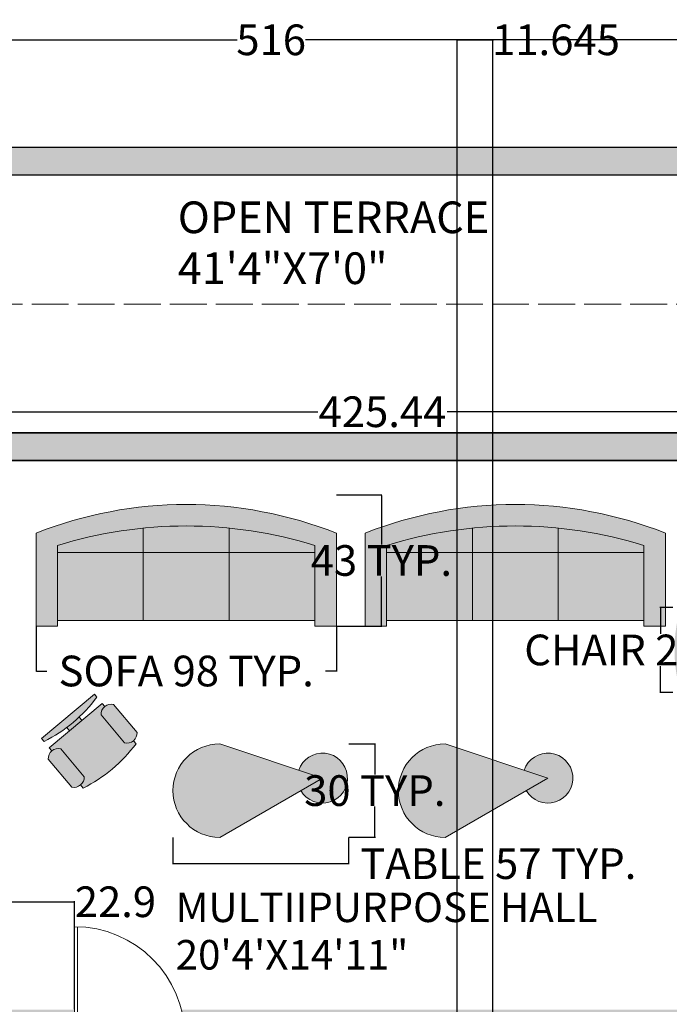
# Model space of a CAD drawing. Units: inches. Extents: x 409 to 1056, y 160 to 945.
# Tile 5 of 6: x 632 to 843, y 624 to 945. Entities that reach past the tile are written whole.
import ezdxf

# ---------------------------------------------------------------- set-up
doc = ezdxf.new("R2010")
doc.units = ezdxf.units.IN
doc.header["$MEASUREMENT"] = 0
doc.linetypes.add('ACAD_ISO02W100', pattern=[15, 12, -3])
for name, color, linetype, lineweight in [('A-ANNO-DIMS', 2, 'Continuous', 18), ('A-AREA-IDEN', 7, 'Continuous', 18), ('A-DOOR', 3, 'Continuous', 18), ('A-FURN', 8, 'Continuous', 18), ('A-ROOF-BYND', 8, 'ACAD_ISO02W100', 13), ('A-WALL', 7, 'Continuous', 35), ('A-WALL-PRPT', 7, 'Continuous', 30)]:
    doc.layers.add(name, color=color, linetype=linetype, lineweight=lineweight)
doc.layers.add('A-FURN-PATT', color=51, linetype='Continuous', lineweight=13, true_color=0xf8f6b0)
doc.layers.add('A-WALL-PATT', color=251, linetype='Continuous', lineweight=13, true_color=0x636466)
doc.styles.get("Standard").update_dxf_attribs({"font": 'arial.ttf'})
doc.dimstyles.get("Standard").update_dxf_attribs({"dimtxt": 10, "dimasz": 0.18, "dimexe": 0.18, "dimexo": 0.0625, "dimgap": 0.09, "dimtad": 0, "dimtih": 1, "dimtoh": 1, "dimdec": 0, "dimzin": 0, "dimdsep": 46, "dimlunit": 3, "dimtxsty": 'Standard', "dimcen": 0.09, "dimadec": 0, "dimazin": 0, "dimtfac": 1, "dimtdec": 0, "dimtofl": 0, "dimtmove": 0, "dimatfit": 3, "dimfxl": 1, "dimtolj": 1, "dimtzin": 0, "dimarcsym": 0})

# ---------------------------------------------------------------- blocks, each defined once
blk = doc.blocks.new('Sofa - Roundback 7 ft.')
for p, q in [((-12.00002, -32.4421), (-12.00003, -6.5971)), ((11.99997, -32.4421), (11.99998, -6.5971)), ((-36.000027, -34), (-36.000027, -11.4696)), ((-35.999844, -13.3819), (35.9998, -13.3819)), ((35.99998, -34), (35.99998, -11.4696)), ((-36.000027, -32.4421), (35.99998, -32.4421))]:
    blk.add_line(p, q)
for points in [[(-36.000027, -34), (-42.000027, -34), (-42.000027, -8)], [(41.99998, -8), (41.99998, -34), (35.99998, -34)]]:
    blk.add_lwpolyline(points)
for centre, radius, start, end in [((0, -114.25), 114.25, 68.43141, 111.5686), ((-0.00001, -127.1968), 121.1968, 72.72033, 107.2797)]:
    blk.add_arc(centre, radius, start, end)
blk = doc.blocks.new('Chair - Desk')
for p, q in [((-8.5, 0), (-8.5, -1)), ((-8.5, 0), (8.5, 0)), ((8.5, 0), (8.5, -1)), ((-2, -3), (-2, -1.9355)), ((2, -1.9576), (2, -3)), ((-8.5, -3), (-8.5, -4)), ((-8.5, -3), (8.5, -3)), ((8.5, -3), (8.5, -4)), ((-10.5, -5), (-10.5, -14)), ((-6.5, -14), (-6.5, -5)), ((6.5, -5), (6.5, -14)), ((10.5, -14), (10.5, -5)), ((-8.5, -15), (-8.5, -16)), ((8.5, -15), (8.5, -16))]:
    blk.add_line(p, q)
for centre, radius, start, end in [((0, 34.625), 36.625, 256.5803, 283.4197), ((-8.5, -6.5), 2.5, 36.8699, 143.1301), ((8.5, -6.5), 2.5, 36.8699, 143.1301), ((-8.5, -12.5), 2.5, 216.8699, 323.1301), ((8.5, -12.5), 2.5, 216.8699, 323.1301), ((0, 19.625), 36.625, 256.5803, 283.4197)]:
    blk.add_arc(centre, radius, start, end)
blk = doc.blocks.new('DOOR-SWING-36IN')
for p, q in [((35, 36), (35, 0)), ((36, 36), (36, 0))]:
    blk.add_line(p, q)
blk.add_arc((36, 36), 36, 180, 270)
blk = doc.blocks.new('TABLE-HALL-ACCENT')
for q in [(15.23, 30.46), (15.23, 0)]:
    blk.add_line((48.7, 19.32), q)
for centre, radius, start, end in [((15.23, 15.23), 15.23, 90, 270), ((48.7, 19.32), 8.14, 210, 161.5857)]:
    blk.add_arc(centre, radius, start, end)
blk = doc.blocks.new('*D19')
at = {"layer": 'A-ANNO-DIMS', "color": 0, "lineweight": -2, "transparency": 16777216}
for p, q in [((844.66, 753.84), (840.37, 753.84)), ((840.55, 753.66), (840.55, 745.22)), ((840.55, 726.25), (840.55, 734.7)), ((844.66, 726.07), (840.37, 726.07))]:
    blk.add_line(p, q, dxfattribs=at)
at = {"layer": 'A-ANNO-DIMS', "color": 0, "transparency": 16777216}
for points in [[(840.52, 753.66), (840.58, 753.66), (840.55, 753.84)], [(840.52, 726.25), (840.58, 726.25), (840.55, 726.07)]]:
    blk.add_solid(points, dxfattribs=at)
at = {"layer": 'Defpoints', "color": 0, "transparency": 16777216}
for p in [(844.72, 753.84), (840.55, 726.07), (844.72, 726.07)]:
    blk.add_point(p, dxfattribs=at)
at = {"layer": 'A-ANNO-DIMS', "color": 0, "transparency": 16777216, "insert": (840.55, 739.96), "char_height": 10, "attachment_point": 5}
blk.add_mtext('\\A1;CHAIR 28 TYP.', dxfattribs=at)
blk = doc.blocks.new('*D21')
at = {"layer": 'A-ANNO-DIMS', "color": 0, "lineweight": -2, "transparency": 16777216}
for p, q in [((637.14, 747.71), (637.14, 732.92)), ((734.98, 747.71), (734.98, 732.92)), ((637.32, 733.1), (640.69, 733.1)), ((734.8, 733.1), (731.42, 733.1))]:
    blk.add_line(p, q, dxfattribs=at)
at = {"layer": 'A-ANNO-DIMS', "color": 0, "transparency": 16777216}
for points in [[(637.32, 733.13), (637.32, 733.07), (637.14, 733.1)], [(734.8, 733.13), (734.8, 733.07), (734.98, 733.1)]]:
    blk.add_solid(points, dxfattribs=at)
at = {"layer": 'Defpoints', "color": 0, "transparency": 16777216}
for p in [(637.14, 747.77), (734.98, 747.77), (734.98, 733.1)]:
    blk.add_point(p, dxfattribs=at)
at = {"layer": 'A-ANNO-DIMS', "color": 0, "transparency": 16777216, "insert": (686.06, 733.1), "char_height": 10, "attachment_point": 5}
blk.add_mtext('\\A1;SOFA 98 TYP.', dxfattribs=at)
blk = doc.blocks.new('*D22')
at = {"layer": 'A-ANNO-DIMS', "color": 0, "lineweight": -2, "transparency": 16777216}
for p, q in [((735.04, 790.48), (749.83, 790.48)), ((749.65, 790.3), (749.65, 774.33)), ((749.65, 747.95), (749.65, 763.93)), ((735.04, 747.77), (749.83, 747.77))]:
    blk.add_line(p, q, dxfattribs=at)
at = {"layer": 'A-ANNO-DIMS', "color": 0, "transparency": 16777216}
for points in [[(749.62, 790.3), (749.68, 790.3), (749.65, 790.48)], [(749.62, 747.95), (749.68, 747.95), (749.65, 747.77)]]:
    blk.add_solid(points, dxfattribs=at)
at = {"layer": 'Defpoints', "color": 0, "transparency": 16777216}
for p in [(734.98, 790.48), (749.65, 790.48), (734.98, 747.77)]:
    blk.add_point(p, dxfattribs=at)
at = {"layer": 'A-ANNO-DIMS', "color": 0, "transparency": 16777216, "insert": (749.65, 769.13), "char_height": 10, "attachment_point": 5}
blk.add_mtext('\\A1;43 TYP.', dxfattribs=at)
blk = doc.blocks.new('*D23')
at = {"layer": 'A-ANNO-DIMS', "color": 0, "lineweight": -2, "transparency": 16777216}
for p, q in [((681.75, 678.81), (681.75, 670.12)), ((738.93, 678.81), (738.93, 670.12)), ((681.93, 670.3), (738.75, 670.3)), ((738.93, 670.3), (739.11, 670.3))]:
    blk.add_line(p, q, dxfattribs=at)
at = {"layer": 'A-ANNO-DIMS', "color": 0, "transparency": 16777216}
for points in [[(681.93, 670.33), (681.93, 670.27), (681.75, 670.3)], [(738.75, 670.33), (738.75, 670.27), (738.93, 670.3)]]:
    blk.add_solid(points, dxfattribs=at)
at = {"layer": 'Defpoints', "color": 0, "transparency": 16777216}
for p in [(681.75, 678.88), (738.93, 678.88), (738.93, 670.3)]:
    blk.add_point(p, dxfattribs=at)
at = {"layer": 'A-ANNO-DIMS', "color": 0, "transparency": 16777216, "insert": (787.74, 670.3), "char_height": 10, "attachment_point": 5}
blk.add_mtext('\\A1;TABLE 57 TYP.', dxfattribs=at)
blk = doc.blocks.new('*D24')
at = {"layer": 'A-ANNO-DIMS', "color": 0, "lineweight": -2, "transparency": 16777216}
for p, q in [((739, 709.34), (747.69, 709.34)), ((747.51, 709.16), (747.51, 699.31)), ((747.51, 679.06), (747.51, 688.91)), ((739, 678.88), (747.69, 678.88))]:
    blk.add_line(p, q, dxfattribs=at)
at = {"layer": 'A-ANNO-DIMS', "color": 0, "transparency": 16777216}
for points in [[(747.48, 709.16), (747.54, 709.16), (747.51, 709.34)], [(747.48, 679.06), (747.54, 679.06), (747.51, 678.88)]]:
    blk.add_solid(points, dxfattribs=at)
at = {"layer": 'Defpoints', "color": 0, "transparency": 16777216}
for p in [(738.93, 709.34), (747.51, 709.34), (738.93, 678.88)]:
    blk.add_point(p, dxfattribs=at)
at = {"layer": 'A-ANNO-DIMS', "color": 0, "transparency": 16777216, "insert": (747.51, 694.11), "char_height": 10, "attachment_point": 5}
blk.add_mtext('\\A1;30 TYP.', dxfattribs=at)
blk = doc.blocks.new('*D35')
at = {"layer": 'A-ANNO-DIMS', "color": 0, "lineweight": -2, "transparency": 16777216}
for p, q in [((455.74, 903.81), (455.74, 939.05)), ((455.92, 938.87), (702.61, 938.87)), ((971.56, 938.87), (724.88, 938.87)), ((971.74, 903.81), (971.74, 939.05))]:
    blk.add_line(p, q, dxfattribs=at)
at = {"layer": 'A-ANNO-DIMS', "color": 0, "transparency": 16777216}
for points in [[(455.92, 938.9), (455.92, 938.84), (455.74, 938.87)], [(971.56, 938.9), (971.56, 938.84), (971.74, 938.87)]]:
    blk.add_solid(points, dxfattribs=at)
at = {"layer": 'Defpoints', "color": 0, "transparency": 16777216}
for p in [(971.74, 938.87), (455.74, 903.74), (971.74, 903.74)]:
    blk.add_point(p, dxfattribs=at)
at = {"layer": 'A-ANNO-DIMS', "color": 0, "transparency": 16777216, "insert": (713.74, 938.87), "char_height": 10, "attachment_point": 5}
blk.add_mtext('\\A1;516', dxfattribs=at)
blk = doc.blocks.new('*D53')
at = {"layer": 'A-ANNO-DIMS', "color": 0, "lineweight": -2, "transparency": 16777216}
for p, q in [((774.31, 452.81), (774.31, 939.05)), ((774.49, 938.87), (785.78, 938.87)), ((785.96, 452.81), (785.96, 939.05)), ((785.96, 938.87), (786.14, 938.87))]:
    blk.add_line(p, q, dxfattribs=at)
at = {"layer": 'A-ANNO-DIMS', "color": 0, "transparency": 16777216}
for points in [[(774.49, 938.9), (774.49, 938.84), (774.31, 938.87)], [(785.78, 938.9), (785.78, 938.84), (785.96, 938.87)]]:
    blk.add_solid(points, dxfattribs=at)
at = {"layer": 'Defpoints', "color": 0, "transparency": 16777216}
for p in [(785.96, 938.87), (774.31, 452.74), (785.96, 452.74)]:
    blk.add_point(p, dxfattribs=at)
at = {"layer": 'A-ANNO-DIMS', "color": 0, "transparency": 16777216, "insert": (806.55, 938.87), "char_height": 10, "attachment_point": 5}
blk.add_mtext('\\A1;11.645', dxfattribs=at)
blk = doc.blocks.new('*D54')
at = {"layer": 'A-ANNO-DIMS', "color": 0, "lineweight": -2, "transparency": 16777216}
for p, q in [((626.74, 622.81), (626.74, 658.05)), ((649.64, 622.81), (649.64, 658.05)), ((626.92, 657.87), (649.46, 657.87)), ((649.64, 657.87), (649.82, 657.87))]:
    blk.add_line(p, q, dxfattribs=at)
at = {"layer": 'A-ANNO-DIMS', "color": 0, "transparency": 16777216}
for points in [[(626.92, 657.9), (626.92, 657.84), (626.74, 657.87)], [(649.46, 657.9), (649.46, 657.84), (649.64, 657.87)]]:
    blk.add_solid(points, dxfattribs=at)
at = {"layer": 'Defpoints', "color": 0, "transparency": 16777216}
for p in [(649.64, 657.87), (626.74, 622.74), (649.64, 622.74)]:
    blk.add_point(p, dxfattribs=at)
at = {"layer": 'A-ANNO-DIMS', "color": 0, "transparency": 16777216, "insert": (663, 657.87), "char_height": 10, "attachment_point": 5}
blk.add_mtext('\\A1;22.9', dxfattribs=at)
blk = doc.blocks.new('*D60')
at = {"layer": 'A-ANNO-DIMS', "color": 0, "lineweight": -2, "transparency": 16777216}
for p, q in [((537.3, 852.68), (537.3, 817.44)), ((962.74, 852.68), (962.74, 817.44)), ((537.48, 817.62), (728.99, 817.62)), ((962.56, 817.62), (771.05, 817.62))]:
    blk.add_line(p, q, dxfattribs=at)
at = {"layer": 'A-ANNO-DIMS', "color": 0, "transparency": 16777216}
for points in [[(537.48, 817.65), (537.48, 817.59), (537.3, 817.62)], [(962.56, 817.65), (962.56, 817.59), (962.74, 817.62)]]:
    blk.add_solid(points, dxfattribs=at)
at = {"layer": 'Defpoints', "color": 0, "transparency": 16777216}
for p in [(537.3, 852.74), (962.74, 852.74), (537.3, 817.62)]:
    blk.add_point(p, dxfattribs=at)
at = {"layer": 'A-ANNO-DIMS', "color": 0, "transparency": 16777216, "insert": (750.02, 817.62), "char_height": 10, "attachment_point": 5}
blk.add_mtext('\\A1;425.44', dxfattribs=at)

msp = doc.modelspace()

# ---------------------------------------------------------------- hatches: boundary and pattern name
at = {"layer": 'A-FURN-PATT', "transparency": 33554661}
h = msp.add_hatch(color=256, dxfattribs=at)
h.dxf.hatch_style = 1
h.paths.add_polyline_path([(700.0326, 771.7872), (672.0783, 771.7872), (672.0783, 749.5866), (700.0326, 749.5866)], flags=17)
h.paths.add_polyline_path([(727.9869, 771.7872), (700.0326, 771.7872), (700.0326, 749.5866), (727.9869, 749.5866)], flags=17)
h.paths.add_polyline_path([(700.0326, 779.6917), (700.0326, 771.7872), (727.9869, 771.7872), (727.9869, 774.0139, 0.05064665)], flags=17)
h.paths.add_polyline_path([(700.0326, 779.6917, 0.04962821), (672.0783, 779.6917), (672.0783, 771.7872), (700.0326, 771.7872)], flags=17)
h.paths.add_polyline_path([(672.0783, 779.6917, 0.05064665), (644.124, 774.0139), (644.124, 771.7872), (672.0783, 771.7872)], flags=17)
h.paths.add_polyline_path([(672.0783, 771.7872), (644.124, 771.7872), (644.124, 749.5866), (672.0783, 749.5866)], flags=17)
h.paths.add_polyline_path([(637.1355, 778.0558), (637.1355, 747.772), (644.124, 747.772), (644.124, 774.0139, -0.15194781), (727.9869, 774.0139), (727.9869, 771.7872), (727.9869, 749.5866), (727.9869, 747.772), (734.9755, 747.772), (734.9755, 778.0558, 0.19047621)])
h.paths.add_polyline_path([(751.3563, 774.0139, -0.15194781), (835.2192, 774.0139), (835.2192, 747.772), (842.2077, 747.772), (842.2077, 778.0558, 0.19047621), (744.3677, 778.0558), (744.3677, 747.772), (751.3563, 747.772)])
h.paths.add_polyline_path([(779.3105, 771.7872), (751.3563, 771.7872), (751.3563, 749.5866), (779.3106, 749.5866)], flags=17)
h.paths.add_polyline_path([(807.2649, 771.7872), (779.3105, 771.7872), (779.3106, 749.5866), (807.2648, 749.5866)], flags=17)
h.paths.add_polyline_path([(835.2192, 771.7872), (807.2649, 771.7872), (807.2648, 749.5866), (835.2192, 749.5866)], flags=17)
h.paths.add_polyline_path([(835.2192, 774.0139, 0.05064665), (807.2649, 779.6917), (807.2649, 771.7872), (835.2192, 771.7872)], flags=17)
h.paths.add_polyline_path([(807.2649, 779.6917, 0.04962821), (779.3105, 779.6917), (779.3105, 771.7872), (807.2649, 771.7872)], flags=17)
h.paths.add_polyline_path([(779.3105, 779.6917, 0.05064665), (751.3563, 774.0139), (751.3563, 771.7872), (779.3105, 771.7872)], flags=17)
h.paths.add_polyline_path([(863.6721, 751.196), (862.3498, 751.196, -0.23606798), (861.0276, 748.5515), (849.1271, 748.5515, -0.23606798), (847.8048, 751.196), (846.4825, 751.196, 0.11764706), (846.4825, 728.7174), (847.8048, 728.7174, -0.23606798), (849.1271, 731.3619), (861.0276, 731.3619, -0.23606798), (862.3498, 728.7174), (863.6721, 728.7174)])
h.paths.add_polyline_path([(861.0276, 753.8406), (849.1271, 753.8406, 0.5), (849.1271, 748.5515), (861.0276, 748.5515, 0.23606798), (862.3498, 751.196, 0.23606798)])
h.paths.add_polyline_path([(861.0276, 731.3619), (849.1271, 731.3619, 0.23606798), (847.8048, 728.7174, 0.23606798), (849.1271, 726.0728), (861.0276, 726.0728, 0.5)])
h.paths.add_polyline_path([(867.6389, 751.196), (866.3167, 751.196, 0.11764706), (866.3167, 728.7174), (867.6389, 728.7174)])
h.paths.add_polyline_path([(865.0666, 742.6012), (863.6721, 742.6012), (863.6721, 737.3121), (865.0666, 737.3121, -0.02732414)])
h.paths.add_polyline_path([(864.1304, 715.9038), (852.2299, 715.9038, 0.5), (852.2299, 710.6147), (864.1304, 710.6147, 0.5)])
h.paths.add_polyline_path([(866.7749, 713.2593), (865.4527, 713.2593, -0.23606798), (864.1304, 710.6147), (852.2299, 710.6147, -0.23606798), (850.9076, 713.2593), (849.5854, 713.2593, 0.11764706), (849.5854, 690.7806), (850.9076, 690.7806, -0.23606798), (852.2299, 693.4252), (864.1304, 693.4252, -0.23606798), (865.4527, 690.7806), (866.7749, 690.7806)])
h.paths.add_polyline_path([(864.1304, 693.4252), (852.2299, 693.4252, 0.5), (852.2299, 688.1361), (864.1304, 688.1361, 0.5)])
h.paths.add_polyline_path([(868.1695, 704.6645), (866.7749, 704.6645), (866.7749, 699.3754), (868.1695, 699.3754, -0.02732414)])
h.paths.add_polyline_path([(870.7418, 713.2593), (869.4195, 713.2593, 0.11764706), (869.4195, 690.7806), (870.7418, 690.7806)])
h.paths.add_polyline_path([(796.1541, 700.7668), (803.8768, 698.1956), (796.8278, 694.1258, 4.66316556)])
h.paths.add_polyline_path([(722.7253, 700.7668), (730.4481, 698.1956), (723.399, 694.1258, 4.66316556)])
h.paths.add_polyline_path([(669.7198, 709.3627), (668.8708, 710.3764, -0.23606798), (665.9944, 709.692), (658.3533, 718.8153, -0.23606798), (659.5316, 721.527), (658.6826, 722.5407), (641.4498, 708.1074), (642.2988, 707.0937, -0.23606798), (645.1752, 707.7781), (652.8164, 698.6548, -0.23606798), (651.638, 695.9431), (652.487, 694.9294, 0.11764706)])
h.paths.add_polyline_path([(645.1752, 707.7781, 0.5), (641.1204, 704.382), (648.7616, 695.2587, 0.5), (652.8164, 698.6548)])
h.paths.add_polyline_path([(662.4081, 722.2113, 0.5), (658.3533, 718.8153), (665.9944, 709.692, 0.23606798), (668.8708, 710.3764, 0.23606798), (670.0492, 713.0881)])
h.paths.add_polyline_path([(656.9846, 724.5681), (656.1356, 725.5818), (638.9027, 711.1485), (639.7518, 710.1348, 0.11764706)])
h.paths.add_polyline_path([(652.0936, 717.0221), (651.1982, 718.0912, -0.02732414), (647.1434, 714.6951), (648.0388, 713.626)], flags=17)
at = {"layer": 'A-WALL-PATT'}
h = msp.add_hatch(color=256, dxfattribs=at)
h.dxf.hatch_style = 1
h.paths.add_polyline_path([(730.4481, 698.1956), (696.9841, 709.3369, 1), (696.9841, 678.8752)], flags=17)
h.paths.add_polyline_path([(803.8768, 698.1956), (770.4128, 709.3369, 1), (770.4128, 678.8752)], flags=17)
h.paths.add_polyline_path([(464.7418, 894.7439), (466.7418, 894.7439), (962.7418, 894.7439), (962.7418, 810.7439), (971.7418, 810.7439), (971.7418, 903.7439), (455.7418, 903.7439), (455.7418, 201.7439), (971.7418, 201.7439), (971.7418, 240.7439), (962.7418, 240.7439), (962.7418, 210.7439), (464.7418, 210.7439)])
h = msp.add_hatch(color=256, dxfattribs=at)
h.dxf.hatch_style = 1
h.paths.add_polyline_path([(626.7418, 801.7439), (870.7418, 801.7439), (870.7418, 710.7439), (870.7418, 683.9043), (875.7418, 683.9043), (875.7418, 707.7439), (962.7418, 707.7439), (962.7418, 710.7439), (875.7418, 710.7439), (875.7418, 722.7439), (875.7418, 801.7439), (885.6955, 801.7439, -0.06325422), (884.5523, 810.7439), (617.7418, 810.7439), (617.7418, 732.9297), (626.7418, 732.9297)])
h.paths.add_polyline_path([(962.7418, 810.7439), (920.5523, 810.7439), (920.5523, 801.7439), (962.7418, 801.7439)], flags=17)
h.paths.add_polyline_path([(971.7418, 810.7439), (962.7418, 810.7439), (962.7418, 801.7439), (962.7418, 707.7439), (962.7418, 622.7439), (962.7418, 613.7439), (962.7418, 548.7439), (856.7418, 548.7439), (847.7418, 548.7439), (776.7418, 548.7439), (776.7418, 569.8172), (768.7418, 569.8172), (768.7418, 539.7439), (847.7418, 539.7439), (971.7418, 539.7439), (971.7418, 613.7439), (971.7418, 707.7439)])
h.paths.add_polyline_path([(883.2418, 622.7439), (875.7418, 622.7439), (684.4993, 622.7439, -0.06325422), (685.6424, 613.7439), (870.7418, 613.7439), (875.7418, 613.7439), (884.3849, 613.7439, -0.06325422)])
h.paths.add_polyline_path([(649.6424, 622.7439), (626.7418, 622.7439), (626.7418, 613.7439), (649.6424, 613.7439)])
h.paths.add_polyline_path([(626.7418, 652.3165), (617.7418, 652.3165), (617.7418, 613.7439), (626.7418, 613.7439), (626.7418, 622.7439)])
h.paths.add_polyline_path([(776.7418, 613.7439), (768.7418, 613.7439), (768.7418, 590.4138), (776.7418, 590.4138)], flags=17)
h.paths.add_polyline_path([(856.7418, 613.7439), (847.7418, 613.7439), (847.7418, 548.7439), (856.7418, 548.7439)], flags=17)
h.paths.add_polyline_path([(962.7418, 622.7439), (919.2418, 622.7439), (919.2418, 613.7439), (962.7418, 613.7439)], flags=17)
h.paths.add_polyline_path([(971.7418, 539.7439), (962.7418, 539.7439), (962.7418, 452.7439), (687.1506, 452.7439, -0.06325422), (686.0074, 443.7439), (962.7418, 443.7439), (962.7418, 331.7439), (927.6873, 331.7439, -0.02784244), (927.9102, 327.7439), (962.7418, 327.7439), (962.7418, 249.7439), (871.7418, 249.7439), (870.7418, 249.7439), (626.7418, 249.7439), (626.7418, 282.7439), (617.7418, 282.7439), (617.7418, 240.7439), (870.7418, 240.7439), (871.7418, 240.7439), (971.7418, 240.7439), (971.7418, 249.7439), (971.7418, 327.7439), (971.7418, 331.7439), (971.7418, 443.7439), (971.7418, 452.7439)])
h.paths.add_polyline_path([(875.7418, 443.7439), (870.7418, 443.7439), (870.7418, 327.7439), (871.7418, 327.7439), (891.9102, 327.7439), (891.9102, 331.7439), (875.7418, 331.7439)], flags=17)

# ---------------------------------------------------------------- linework, layer by layer
at = {"layer": 'A-ROOF-BYND'}
msp.add_line((962.7418, 852.7439), (537.2978, 852.7439), dxfattribs=at)
at = {"layer": 'A-WALL'}
for p, q in [((884.5523, 810.7439), (617.7418, 810.7439)), ((870.7418, 801.7439), (626.7418, 801.7439))]:
    msp.add_line(p, q, dxfattribs=at)
at = {"layer": 'A-WALL-PRPT'}
for p, q in [((971.7418, 903.7439), (455.7418, 903.7439)), ((962.7418, 894.7439), (466.7418, 894.7439))]:
    msp.add_line(p, q, dxfattribs=at)

# ---------------------------------------------------------------- block references
at = {"layer": 'A-DOOR', "rotation": 180}
msp.add_blockref('DOOR-SWING-36IN', (685.6428, 649.7438), dxfattribs=at)
at = {"layer": 'A-FURN', "xscale": 1.164762366535083, "yscale": 1.164762366535083, "zscale": 1.164762366535083}
for p in [(686.0555, 787.3739), (793.2877, 787.3739)]:
    msp.add_blockref('Sofa - Roundback 7 ft.', p, dxfattribs=at)
at = {"layer": 'A-FURN', "xscale": 1.322274350512927, "yscale": 1.322274350512927, "zscale": 1.322274350512927, "rotation": 39.94772932037304}
msp.add_blockref('Chair - Desk', (647.5192, 718.3651), dxfattribs=at)
at = {"layer": 'A-FURN'}
for p in [(681.753, 678.875), (755.1818, 678.875)]:
    msp.add_blockref('TABLE-HALL-ACCENT', p, dxfattribs=at)

# ---------------------------------------------------------------- texts
at = {"layer": 'A-AREA-IDEN'}
for s, height, p in [('OPEN TERRACE', 10.325829, (683.3142, 875.8379)), ('41\'4"X7\'0"', 10.32583, (683.3142, 859.2504)), ('MULTIIPURPOSE HALL', 9.637213, (682.6286, 651.2524)), ('20\'4\'X14\'11"', 9.637213, (682.6286, 635.7711))]:
    msp.add_text(s, height=height, dxfattribs=at).set_placement(p)

# ---------------------------------------------------------------- dimensions: what is measured, and where the dimension line sits
at = {"layer": 'A-ANNO-DIMS'}
for base, p1, p2, override, picture, middle in [((971.7418, 938.8689), (455.7418, 903.7439), (971.7418, 903.7439), {"dimdec": 0, "dimlfac": 1, "dimrnd": 0, "dimzin": 0, "dimdsep": 46, "dimlunit": 2}, '*D35', (713.7418, 938.8689)), ((785.956, 938.8689), (774.3113, 452.7439), (785.956, 452.7439), {"dimdec": 3, "dimlfac": 1, "dimrnd": 0, "dimzin": 0, "dimdsep": 46, "dimlunit": 2}, '*D53', (806.55, 938.8689)), ((649.6424, 657.8689), (626.7418, 622.7439), (649.6424, 622.7439), {"dimdec": 1, "dimlfac": 1, "dimrnd": 0, "dimzin": 0, "dimdsep": 46, "dimlunit": 2}, '*D54', (662.9956, 657.8689))]:
    dim = msp.add_linear_dim(base=base, p1=p1, p2=p2, dimstyle='Standard', override=override, dxfattribs=at)
    dim.commit()
    dim.dimension.update_dxf_attribs({"geometry": picture, "text_midpoint": middle})
dim = msp.add_linear_dim(base=(537.2978, 817.6189), p1=(962.7418, 852.7439), p2=(537.2978, 852.7439), angle=180, dimstyle='Standard', override={"dimdec": 2, "dimlfac": 1, "dimrnd": 0, "dimzin": 0, "dimdsep": 46, "dimlunit": 2}, dxfattribs=at)
dim.commit()
dim.dimension.update_dxf_attribs({"geometry": '*D60', "text_midpoint": (750.0198, 817.6189)})
for base, p1, p2, angle, text, picture, middle in [((749.6515, 790.4799), (734.9755, 747.772), (734.9755, 790.4799), 90, '<> TYP.', '*D22', (749.6515, 769.126)), ((840.5543, 726.0728), (844.7195, 753.8406), (844.7195, 726.0728), 270, 'CHAIR <> TYP.', '*D19', (840.5543, 739.9567)), ((747.5104, 709.3369), (738.9334, 678.8752), (738.9334, 709.3369), 90, '<> TYP.', '*D24', (747.5104, 694.106))]:
    dim = msp.add_linear_dim(base=base, p1=p1, p2=p2, angle=angle, text=text, dimstyle='Standard', override={"dimdec": 0, "dimlfac": 1, "dimrnd": 0, "dimzin": 0, "dimdsep": 46, "dimlunit": 2}, dxfattribs=at)
    dim.commit()
    dim.dimension.update_dxf_attribs({"geometry": picture, "text_midpoint": middle})
for base, p1, p2, text, picture, middle in [((734.9755, 733.096), (637.1355, 747.772), (734.9755, 747.772), 'SOFA <> TYP.', '*D21', (686.0555, 733.096)), ((738.9334, 670.2981), (681.7532, 678.8752), (738.9334, 678.8752), 'TABLE <> TYP.', '*D23', (787.7368, 670.2981))]:
    dim = msp.add_linear_dim(base=base, p1=p1, p2=p2, text=text, dimstyle='Standard', override={"dimdec": 0, "dimlfac": 1, "dimrnd": 0, "dimzin": 0, "dimdsep": 46, "dimlunit": 2}, dxfattribs=at)
    dim.commit()
    dim.dimension.update_dxf_attribs({"geometry": picture, "text_midpoint": middle})

doc.saveas('drawing.dxf')
